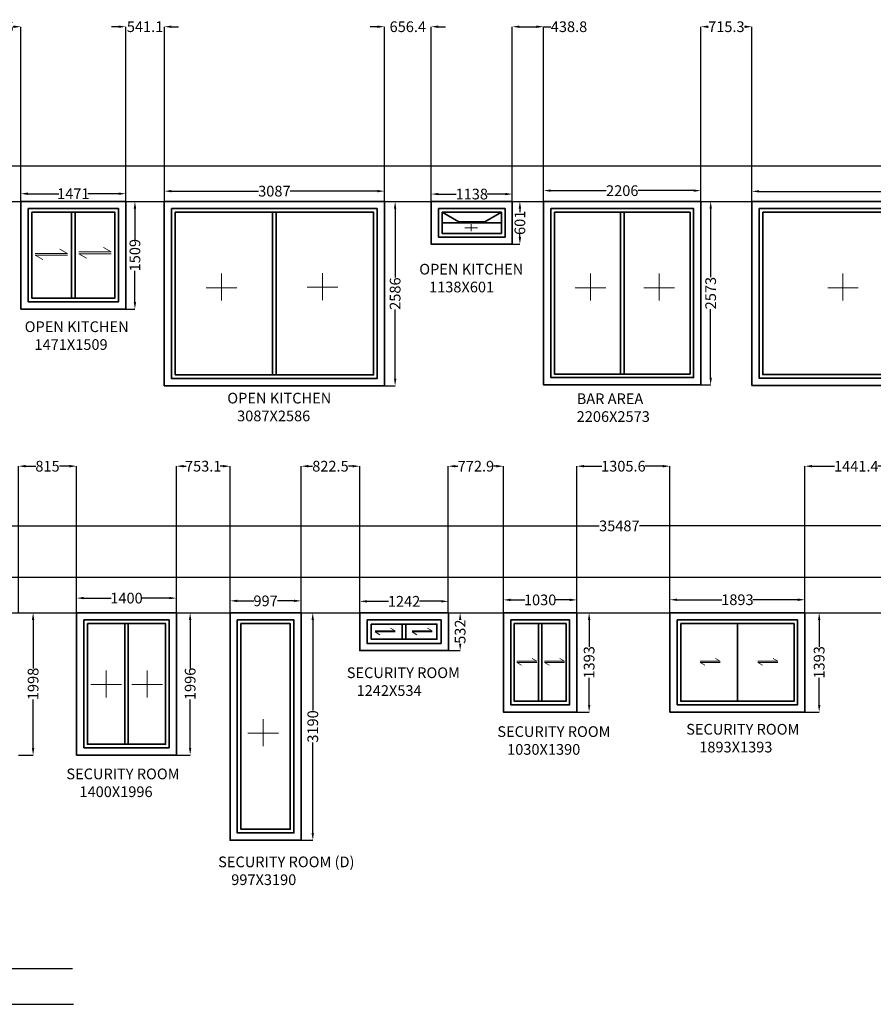
# Model space of a CAD drawing. Units: millimetres. Extents: x 16338 to 57165, y -4429 to 26237.
# Tile 5 of 6: x 28512 to 40486, y 12430 to 26237. Entities that reach past the tile are written whole.
import ezdxf

# ---------------------------------------------------------------- set-up
doc = ezdxf.new("R2010")
doc.units = ezdxf.units.MM
doc.header["$MEASUREMENT"] = 0
for name, color, linetype, lineweight in [('A-ANNO-DIMS', 5, 'Continuous', 18), ('A-ANNO-SYMB', 4, 'Continuous', 18), ('A-ANNO-TEXT', 3, 'Continuous', 18), ('A-ELEV', 8, 'Continuous', 25), ('A-GLAZ', 7, 'Continuous', 35)]:
    doc.layers.add(name, color=color, linetype=linetype, lineweight=lineweight)
doc.styles.get("Standard").update_dxf_attribs({"font": 'arial.ttf'})
doc.dimstyles.get("Standard").update_dxf_attribs({"dimtxt": 150, "dimasz": 100, "dimexe": 0.18, "dimexo": 0.0625, "dimgap": 0.09, "dimtad": 0, "dimdec": 0, "dimzin": 0, "dimdsep": 46, "dimtxsty": 'Standard', "dimcen": 0.09, "dimadec": 0, "dimazin": 0, "dimtfac": 1, "dimtdec": 0, "dimtofl": 0, "dimtmove": 0, "dimatfit": 3, "dimfxl": 1, "dimtolj": 1, "dimtzin": 0, "dimarcsym": 0})

# ---------------------------------------------------------------- blocks, each defined once
blk = doc.blocks.new('*D6')
at = {"layer": 'A-ANNO-DIMS', "color": 0, "lineweight": -2, "transparency": 16777216}
for p, q in [((28528, 23689), (28528, 23797)), ((28628, 23797), (29061, 23797)), ((29899, 23797), (29466, 23797)), ((29999, 23689), (29999, 23797))]:
    blk.add_line(p, q, dxfattribs=at)
at = {"layer": 'A-ANNO-DIMS', "color": 0, "transparency": 16777216}
for points in [[(28628, 23814), (28628, 23780), (28528, 23797)], [(29899, 23814), (29899, 23780), (29999, 23797)]]:
    blk.add_solid(points, dxfattribs=at)
at = {"layer": 'Defpoints', "color": 0, "transparency": 16777216}
for p in [(29999, 23797), (28528, 23689), (29999, 23689)]:
    blk.add_point(p, dxfattribs=at)
at = {"layer": 'A-ANNO-DIMS', "color": 0, "transparency": 16777216, "insert": (29264, 23797), "char_height": 150, "attachment_point": 5}
blk.add_mtext('\\A1;1471', dxfattribs=at)
blk = doc.blocks.new('*D7')
at = {"layer": 'A-ANNO-DIMS', "color": 0, "lineweight": -2, "transparency": 16777216}
for p, q in [((29999, 23689), (30128, 23689)), ((30128, 23589), (30128, 23152)), ((30128, 22280), (30128, 22717)), ((29999, 22180), (30128, 22180))]:
    blk.add_line(p, q, dxfattribs=at)
at = {"layer": 'A-ANNO-DIMS', "color": 0, "transparency": 16777216}
for points in [[(30111, 23589), (30145, 23589), (30128, 23689)], [(30111, 22280), (30145, 22280), (30128, 22180)]]:
    blk.add_solid(points, dxfattribs=at)
at = {"layer": 'Defpoints', "color": 0, "transparency": 16777216}
for p in [(29999, 23689), (29999, 22180), (30128, 22180)]:
    blk.add_point(p, dxfattribs=at)
at = {"layer": 'A-ANNO-DIMS', "color": 0, "transparency": 16777216, "insert": (30128, 22935), "char_height": 150, "attachment_point": 5, "rotation": 90}
blk.add_mtext('\\A1;1509', dxfattribs=at)
blk = doc.blocks.new('*D8')
at = {"layer": 'A-ANNO-DIMS', "color": 0, "lineweight": -2, "transparency": 16777216}
for p, q in [((30541, 23689), (30541, 23833)), ((30641, 23833), (31860, 23833)), ((33528, 23833), (32308, 23833)), ((33628, 23689), (33628, 23833))]:
    blk.add_line(p, q, dxfattribs=at)
at = {"layer": 'A-ANNO-DIMS', "color": 0, "transparency": 16777216}
for points in [[(30641, 23850), (30641, 23816), (30541, 23833)], [(33528, 23850), (33528, 23816), (33628, 23833)]]:
    blk.add_solid(points, dxfattribs=at)
at = {"layer": 'Defpoints', "color": 0, "transparency": 16777216}
for p in [(33628, 23833), (30541, 23689), (33628, 23689)]:
    blk.add_point(p, dxfattribs=at)
at = {"layer": 'A-ANNO-DIMS', "color": 0, "transparency": 16777216, "insert": (32084, 23833), "char_height": 150, "attachment_point": 5}
blk.add_mtext('\\A1;3087', dxfattribs=at)
blk = doc.blocks.new('*D9')
at = {"layer": 'A-ANNO-DIMS', "color": 0, "lineweight": -2, "transparency": 16777216}
for p, q in [((33628, 23689), (33779, 23689)), ((33778, 23589), (33778, 22621)), ((33778, 21203), (33778, 22171)), ((33628, 21103), (33779, 21103))]:
    blk.add_line(p, q, dxfattribs=at)
at = {"layer": 'A-ANNO-DIMS', "color": 0, "transparency": 16777216}
for points in [[(33762, 23589), (33795, 23589), (33778, 23689)], [(33762, 21203), (33795, 21203), (33778, 21103)]]:
    blk.add_solid(points, dxfattribs=at)
at = {"layer": 'Defpoints', "color": 0, "transparency": 16777216}
for p in [(33628, 23689), (33628, 21103), (33778, 21103)]:
    blk.add_point(p, dxfattribs=at)
at = {"layer": 'A-ANNO-DIMS', "color": 0, "transparency": 16777216, "insert": (33778, 22396), "char_height": 150, "attachment_point": 5, "rotation": 90}
blk.add_mtext('\\A1;2586', dxfattribs=at)
blk = doc.blocks.new('*D10')
at = {"layer": 'A-ANNO-DIMS', "color": 0, "lineweight": -2, "transparency": 16777216}
for p, q in [((34284, 23689), (34284, 23792)), ((34384, 23792), (34636, 23792)), ((35322, 23792), (35070, 23792)), ((35422, 23689), (35422, 23792))]:
    blk.add_line(p, q, dxfattribs=at)
at = {"layer": 'A-ANNO-DIMS', "color": 0, "transparency": 16777216}
for points in [[(34384, 23809), (34384, 23775), (34284, 23792)], [(35322, 23809), (35322, 23775), (35422, 23792)]]:
    blk.add_solid(points, dxfattribs=at)
at = {"layer": 'Defpoints', "color": 0, "transparency": 16777216}
for p in [(35422, 23792), (34284, 23689), (35422, 23689)]:
    blk.add_point(p, dxfattribs=at)
at = {"layer": 'A-ANNO-DIMS', "color": 0, "transparency": 16777216, "insert": (34853, 23792), "char_height": 150, "attachment_point": 5}
blk.add_mtext('\\A1;1138', dxfattribs=at)
blk = doc.blocks.new('*D11')
at = {"layer": 'A-ANNO-DIMS', "color": 0, "lineweight": -2, "transparency": 16777216}
for p, q in [((35422, 23689), (35528, 23689)), ((35528, 23589), (35528, 23540)), ((35528, 23188), (35528, 23237)), ((35422, 23088), (35528, 23088))]:
    blk.add_line(p, q, dxfattribs=at)
at = {"layer": 'A-ANNO-DIMS', "color": 0, "transparency": 16777216}
for points in [[(35511, 23589), (35545, 23589), (35528, 23689)], [(35511, 23188), (35545, 23188), (35528, 23088)]]:
    blk.add_solid(points, dxfattribs=at)
at = {"layer": 'Defpoints', "color": 0, "transparency": 16777216}
for p in [(35422, 23689), (35422, 23088), (35528, 23088)]:
    blk.add_point(p, dxfattribs=at)
at = {"layer": 'A-ANNO-DIMS', "color": 0, "transparency": 16777216, "insert": (35528, 23389), "char_height": 150, "attachment_point": 5, "rotation": 90}
blk.add_mtext('\\A1;601', dxfattribs=at)
blk = doc.blocks.new('*D12')
at = {"layer": 'A-ANNO-DIMS', "color": 0, "lineweight": -2, "transparency": 16777216}
for p, q in [((35861, 23689), (35861, 23840)), ((35961, 23840), (36738, 23840)), ((37967, 23840), (37189, 23840)), ((38067, 23689), (38067, 23840))]:
    blk.add_line(p, q, dxfattribs=at)
at = {"layer": 'A-ANNO-DIMS', "color": 0, "transparency": 16777216}
for points in [[(35961, 23857), (35961, 23824), (35861, 23840)], [(37967, 23857), (37967, 23824), (38067, 23840)]]:
    blk.add_solid(points, dxfattribs=at)
at = {"layer": 'Defpoints', "color": 0, "transparency": 16777216}
for p in [(38067, 23840), (35861, 23689), (38067, 23689)]:
    blk.add_point(p, dxfattribs=at)
at = {"layer": 'A-ANNO-DIMS', "color": 0, "transparency": 16777216, "insert": (36964, 23840), "char_height": 150, "attachment_point": 5}
blk.add_mtext('\\A1;2206', dxfattribs=at)
blk = doc.blocks.new('*D13')
at = {"layer": 'A-ANNO-DIMS', "color": 0, "lineweight": -2, "transparency": 16777216}
for p, q in [((38067, 23689), (38205, 23689)), ((38204, 23589), (38204, 22628)), ((38204, 21216), (38204, 22177)), ((38067, 21116), (38205, 21116))]:
    blk.add_line(p, q, dxfattribs=at)
at = {"layer": 'A-ANNO-DIMS', "color": 0, "transparency": 16777216}
for points in [[(38188, 23589), (38221, 23589), (38204, 23689)], [(38188, 21216), (38221, 21216), (38204, 21116)]]:
    blk.add_solid(points, dxfattribs=at)
at = {"layer": 'Defpoints', "color": 0, "transparency": 16777216}
for p in [(38067, 23689), (38067, 21116), (38204, 21116)]:
    blk.add_point(p, dxfattribs=at)
at = {"layer": 'A-ANNO-DIMS', "color": 0, "transparency": 16777216, "insert": (38204, 22403), "char_height": 150, "attachment_point": 5, "rotation": 90}
blk.add_mtext('\\A1;2573', dxfattribs=at)
blk = doc.blocks.new('*D14')
at = {"layer": 'A-ANNO-DIMS', "color": 0, "lineweight": -2, "transparency": 16777216}
for p, q in [((38782, 23689), (38782, 23831)), ((38882, 23830), (41002, 23830)), ((43575, 23830), (41456, 23830)), ((43675, 23689), (43675, 23831))]:
    blk.add_line(p, q, dxfattribs=at)
at = {"layer": 'A-ANNO-DIMS', "color": 0, "transparency": 16777216}
for points in [[(38882, 23847), (38882, 23814), (38782, 23830)], [(43575, 23847), (43575, 23814), (43675, 23830)]]:
    blk.add_solid(points, dxfattribs=at)
at = {"layer": 'Defpoints', "color": 0, "transparency": 16777216}
for p in [(43675, 23830), (38782, 23689), (43675, 23689)]:
    blk.add_point(p, dxfattribs=at)
at = {"layer": 'A-ANNO-DIMS', "color": 0, "transparency": 16777216, "insert": (41229, 23830), "char_height": 150, "attachment_point": 5}
blk.add_mtext('\\A1;4893', dxfattribs=at)
blk = doc.blocks.new('*D25')
at = {"layer": 'A-ANNO-DIMS', "color": 0, "lineweight": -2, "transparency": 16777216}
for p, q in [((28495, 17921), (28700, 17921)), ((28700, 17821), (28700, 17139)), ((28700, 16023), (28700, 16705)), ((28495, 15923), (28700, 15923))]:
    blk.add_line(p, q, dxfattribs=at)
at = {"layer": 'A-ANNO-DIMS', "color": 0, "transparency": 16777216}
for points in [[(28683, 17821), (28717, 17821), (28700, 17921)], [(28683, 16023), (28717, 16023), (28700, 15923)]]:
    blk.add_solid(points, dxfattribs=at)
at = {"layer": 'Defpoints', "color": 0, "transparency": 16777216}
for p in [(28495, 17921), (28495, 15923), (28700, 15923)]:
    blk.add_point(p, dxfattribs=at)
at = {"layer": 'A-ANNO-DIMS', "color": 0, "transparency": 16777216, "insert": (28700, 16922), "char_height": 150, "attachment_point": 5, "rotation": 90}
blk.add_mtext('\\A1;1998', dxfattribs=at)
blk = doc.blocks.new('*D26')
at = {"layer": 'A-ANNO-DIMS', "color": 0, "lineweight": -2, "transparency": 16777216}
for p, q in [((29310, 17921), (29310, 18127)), ((29410, 18126), (29793, 18126)), ((30610, 18126), (30227, 18126)), ((30710, 17921), (30710, 18127))]:
    blk.add_line(p, q, dxfattribs=at)
at = {"layer": 'A-ANNO-DIMS', "color": 0, "transparency": 16777216}
for points in [[(29410, 18143), (29410, 18110), (29310, 18126)], [(30610, 18143), (30610, 18110), (30710, 18126)]]:
    blk.add_solid(points, dxfattribs=at)
at = {"layer": 'Defpoints', "color": 0, "transparency": 16777216}
for p in [(30710, 18126), (29310, 17921), (30710, 17921)]:
    blk.add_point(p, dxfattribs=at)
at = {"layer": 'A-ANNO-DIMS', "color": 0, "transparency": 16777216, "insert": (30010, 18126), "char_height": 150, "attachment_point": 5}
blk.add_mtext('\\A1;1400', dxfattribs=at)
blk = doc.blocks.new('*D27')
at = {"layer": 'A-ANNO-DIMS', "color": 0, "lineweight": -2, "transparency": 16777216}
for p, q in [((30710, 17921), (30903, 17921)), ((30903, 17821), (30903, 17140)), ((30903, 16025), (30903, 16706)), ((30710, 15925), (30903, 15925))]:
    blk.add_line(p, q, dxfattribs=at)
at = {"layer": 'A-ANNO-DIMS', "color": 0, "transparency": 16777216}
for points in [[(30886, 17821), (30919, 17821), (30903, 17921)], [(30886, 16025), (30919, 16025), (30903, 15925)]]:
    blk.add_solid(points, dxfattribs=at)
at = {"layer": 'Defpoints', "color": 0, "transparency": 16777216}
for p in [(30710, 17921), (30710, 15925), (30903, 15925)]:
    blk.add_point(p, dxfattribs=at)
at = {"layer": 'A-ANNO-DIMS', "color": 0, "transparency": 16777216, "insert": (30903, 16923), "char_height": 150, "attachment_point": 5, "rotation": 90}
blk.add_mtext('\\A1;1996', dxfattribs=at)
blk = doc.blocks.new('*D28')
at = {"layer": 'A-ANNO-DIMS', "color": 0, "lineweight": -2, "transparency": 16777216}
for p, q in [((31463, 17921), (31463, 18087)), ((31563, 18087), (31796, 18087)), ((32360, 18087), (32127, 18087)), ((32460, 17921), (32460, 18087))]:
    blk.add_line(p, q, dxfattribs=at)
at = {"layer": 'A-ANNO-DIMS', "color": 0, "transparency": 16777216}
for points in [[(31563, 18104), (31563, 18071), (31463, 18087)], [(32360, 18104), (32360, 18071), (32460, 18087)]]:
    blk.add_solid(points, dxfattribs=at)
at = {"layer": 'Defpoints', "color": 0, "transparency": 16777216}
for p in [(32460, 18087), (31463, 17921), (32460, 17921)]:
    blk.add_point(p, dxfattribs=at)
at = {"layer": 'A-ANNO-DIMS', "color": 0, "transparency": 16777216, "insert": (31961, 18087), "char_height": 150, "attachment_point": 5}
blk.add_mtext('\\A1;997', dxfattribs=at)
blk = doc.blocks.new('*D29')
at = {"layer": 'A-ANNO-DIMS', "color": 0, "lineweight": -2, "transparency": 16777216}
for p, q in [((32460, 17921), (32623, 17921)), ((32623, 17821), (32623, 16550)), ((32623, 14831), (32623, 16102)), ((32460, 14731), (32623, 14731))]:
    blk.add_line(p, q, dxfattribs=at)
at = {"layer": 'A-ANNO-DIMS', "color": 0, "transparency": 16777216}
for points in [[(32606, 17821), (32639, 17821), (32623, 17921)], [(32606, 14831), (32639, 14831), (32623, 14731)]]:
    blk.add_solid(points, dxfattribs=at)
at = {"layer": 'Defpoints', "color": 0, "transparency": 16777216}
for p in [(32460, 17921), (32460, 14731), (32623, 14731)]:
    blk.add_point(p, dxfattribs=at)
at = {"layer": 'A-ANNO-DIMS', "color": 0, "transparency": 16777216, "insert": (32623, 16326), "char_height": 150, "attachment_point": 5, "rotation": 90}
blk.add_mtext('\\A1;3190', dxfattribs=at)
blk = doc.blocks.new('*D30')
at = {"layer": 'A-ANNO-DIMS', "color": 0, "lineweight": -2, "transparency": 16777216}
for p, q in [((33282, 17921), (33282, 18081)), ((33382, 18081), (33687, 18081)), ((34424, 18081), (34120, 18081)), ((34524, 17921), (34524, 18081))]:
    blk.add_line(p, q, dxfattribs=at)
at = {"layer": 'A-ANNO-DIMS', "color": 0, "transparency": 16777216}
for points in [[(33382, 18097), (33382, 18064), (33282, 18081)], [(34424, 18097), (34424, 18064), (34524, 18081)]]:
    blk.add_solid(points, dxfattribs=at)
at = {"layer": 'Defpoints', "color": 0, "transparency": 16777216}
for p in [(34524, 18081), (33282, 17921), (34524, 17921)]:
    blk.add_point(p, dxfattribs=at)
at = {"layer": 'A-ANNO-DIMS', "color": 0, "transparency": 16777216, "insert": (33903, 18081), "char_height": 150, "attachment_point": 5}
blk.add_mtext('\\A1;1242', dxfattribs=at)
blk = doc.blocks.new('*D31')
at = {"layer": 'A-ANNO-DIMS', "color": 0, "lineweight": -2, "transparency": 16777216}
for p, q in [((34525, 17921), (34690, 17921)), ((34690, 17821), (34690, 17820)), ((34690, 17489), (34690, 17490)), ((34525, 17389), (34690, 17389))]:
    blk.add_line(p, q, dxfattribs=at)
at = {"layer": 'A-ANNO-DIMS', "color": 0, "transparency": 16777216}
for points in [[(34674, 17821), (34707, 17821), (34690, 17921)], [(34674, 17489), (34707, 17489), (34690, 17389)]]:
    blk.add_solid(points, dxfattribs=at)
at = {"layer": 'Defpoints', "color": 0, "transparency": 16777216}
for p in [(34524, 17921), (34524, 17389), (34690, 17389)]:
    blk.add_point(p, dxfattribs=at)
at = {"layer": 'A-ANNO-DIMS', "color": 0, "transparency": 16777216, "insert": (34690, 17655), "char_height": 150, "attachment_point": 5, "rotation": 90}
blk.add_mtext('\\A1;532', dxfattribs=at)
blk = doc.blocks.new('*D32')
at = {"layer": 'A-ANNO-DIMS', "color": 0, "lineweight": -2, "transparency": 16777216}
for p, q in [((35297, 17921), (35297, 18101)), ((35397, 18101), (35596, 18101)), ((36227, 18101), (36029, 18101)), ((36327, 17921), (36327, 18101))]:
    blk.add_line(p, q, dxfattribs=at)
at = {"layer": 'A-ANNO-DIMS', "color": 0, "transparency": 16777216}
for points in [[(35397, 18118), (35397, 18084), (35297, 18101)], [(36227, 18118), (36227, 18084), (36327, 18101)]]:
    blk.add_solid(points, dxfattribs=at)
at = {"layer": 'Defpoints', "color": 0, "transparency": 16777216}
for p in [(36327, 18101), (35297, 17921), (36327, 17921)]:
    blk.add_point(p, dxfattribs=at)
at = {"layer": 'A-ANNO-DIMS', "color": 0, "transparency": 16777216, "insert": (35812, 18101), "char_height": 150, "attachment_point": 5}
blk.add_mtext('\\A1;1030', dxfattribs=at)
blk = doc.blocks.new('*D33')
at = {"layer": 'A-ANNO-DIMS', "color": 0, "lineweight": -2, "transparency": 16777216}
for p, q in [((36327, 17921), (36500, 17921)), ((36499, 17821), (36499, 17442)), ((36499, 16628), (36499, 17008)), ((36327, 16528), (36500, 16528))]:
    blk.add_line(p, q, dxfattribs=at)
at = {"layer": 'A-ANNO-DIMS', "color": 0, "transparency": 16777216}
for points in [[(36483, 17821), (36516, 17821), (36499, 17921)], [(36483, 16628), (36516, 16628), (36499, 16528)]]:
    blk.add_solid(points, dxfattribs=at)
at = {"layer": 'Defpoints', "color": 0, "transparency": 16777216}
for p in [(36327, 17921), (36327, 16528), (36499, 16528)]:
    blk.add_point(p, dxfattribs=at)
at = {"layer": 'A-ANNO-DIMS', "color": 0, "transparency": 16777216, "insert": (36499, 17225), "char_height": 150, "attachment_point": 5, "rotation": 90}
blk.add_mtext('\\A1;1393', dxfattribs=at)
blk = doc.blocks.new('*D34')
at = {"layer": 'A-ANNO-DIMS', "color": 0, "lineweight": -2, "transparency": 16777216}
for p, q in [((37633, 17921), (37633, 18103)), ((37733, 18103), (38362, 18103)), ((39426, 18103), (38796, 18103)), ((39526, 17921), (39526, 18103))]:
    blk.add_line(p, q, dxfattribs=at)
at = {"layer": 'A-ANNO-DIMS', "color": 0, "transparency": 16777216}
for points in [[(37733, 18120), (37733, 18086), (37633, 18103)], [(39426, 18120), (39426, 18086), (39526, 18103)]]:
    blk.add_solid(points, dxfattribs=at)
at = {"layer": 'Defpoints', "color": 0, "transparency": 16777216}
for p in [(39526, 18103), (37633, 17921), (39526, 17921)]:
    blk.add_point(p, dxfattribs=at)
at = {"layer": 'A-ANNO-DIMS', "color": 0, "transparency": 16777216, "insert": (38579, 18103), "char_height": 150, "attachment_point": 5}
blk.add_mtext('\\A1;1893', dxfattribs=at)
blk = doc.blocks.new('*D35')
at = {"layer": 'A-ANNO-DIMS', "color": 0, "lineweight": -2, "transparency": 16777216}
for p, q in [((39526, 17921), (39726, 17921)), ((39726, 17821), (39726, 17442)), ((39726, 16628), (39726, 17008)), ((39526, 16528), (39726, 16528))]:
    blk.add_line(p, q, dxfattribs=at)
at = {"layer": 'A-ANNO-DIMS', "color": 0, "transparency": 16777216}
for points in [[(39710, 17821), (39743, 17821), (39726, 17921)], [(39710, 16628), (39743, 16628), (39726, 16528)]]:
    blk.add_solid(points, dxfattribs=at)
at = {"layer": 'Defpoints', "color": 0, "transparency": 16777216}
for p in [(39526, 17921), (39526, 16528), (39726, 16528)]:
    blk.add_point(p, dxfattribs=at)
at = {"layer": 'A-ANNO-DIMS', "color": 0, "transparency": 16777216, "insert": (39726, 17225), "char_height": 150, "attachment_point": 5, "rotation": 90}
blk.add_mtext('\\A1;1393', dxfattribs=at)
blk = doc.blocks.new('SLIDE-ARROW-L')
for p, q in [((454, 0), (347, 62)), ((0, 0), (454, 0))]:
    blk.add_line(p, q)
blk = doc.blocks.new('SLIDE-ARROW-M')
for p, q in [((0, 0), (281, 0)), ((281, 0), (215, 38))]:
    blk.add_line(p, q)
blk = doc.blocks.new('*D84')
at = {"layer": 'A-ANNO-DIMS', "color": 0, "lineweight": -2, "transparency": 16777216}
for p, q in [((27982, 23689), (27982, 26139)), ((28082, 26139), (28090, 26139)), ((28428, 26139), (28421, 26139)), ((28528, 23689), (28528, 26139))]:
    blk.add_line(p, q, dxfattribs=at)
at = {"layer": 'A-ANNO-DIMS', "color": 0, "transparency": 16777216}
for points in [[(28082, 26156), (28082, 26122), (27982, 26139)], [(28428, 26156), (28428, 26122), (28528, 26139)]]:
    blk.add_solid(points, dxfattribs=at)
at = {"layer": 'Defpoints', "color": 0, "transparency": 16777216}
for p in [(28528, 26139), (27982, 23689), (28528, 23689)]:
    blk.add_point(p, dxfattribs=at)
at = {"layer": 'A-ANNO-DIMS', "color": 0, "transparency": 16777216, "insert": (28255, 26139), "char_height": 150, "attachment_point": 5}
blk.add_mtext('\\A1;546', dxfattribs=at)
blk = doc.blocks.new('*D85')
at = {"layer": 'A-ANNO-DIMS', "color": 0, "lineweight": -2, "transparency": 16777216}
for p, q in [((29899, 26139), (29799, 26139)), ((29999, 23689), (29999, 26139)), ((30541, 23689), (30541, 26139)), ((30641, 26139), (30741, 26139))]:
    blk.add_line(p, q, dxfattribs=at)
at = {"layer": 'A-ANNO-DIMS', "color": 0, "transparency": 16777216}
for points in [[(29899, 26156), (29899, 26122), (29999, 26139)], [(30641, 26156), (30641, 26122), (30541, 26139)]]:
    blk.add_solid(points, dxfattribs=at)
at = {"layer": 'Defpoints', "color": 0, "transparency": 16777216}
for p in [(30541, 26139), (29999, 23689), (30541, 23689)]:
    blk.add_point(p, dxfattribs=at)
at = {"layer": 'A-ANNO-DIMS', "color": 0, "transparency": 16777216, "insert": (30270, 26139), "char_height": 150, "attachment_point": 5}
blk.add_mtext('\\A1;541.1', dxfattribs=at)
blk = doc.blocks.new('*D86')
at = {"layer": 'A-ANNO-DIMS', "color": 0, "lineweight": -2, "transparency": 16777216}
for p, q in [((33528, 26139), (33428, 26139)), ((33628, 23689), (33628, 26139)), ((34284, 23689), (34284, 26139)), ((34384, 26139), (34484, 26139))]:
    blk.add_line(p, q, dxfattribs=at)
at = {"layer": 'A-ANNO-DIMS', "color": 0, "transparency": 16777216}
for points in [[(33528, 26156), (33528, 26122), (33628, 26139)], [(34384, 26156), (34384, 26122), (34284, 26139)]]:
    blk.add_solid(points, dxfattribs=at)
at = {"layer": 'Defpoints', "color": 0, "transparency": 16777216}
for p in [(34284, 26139), (33628, 23689), (34284, 23689)]:
    blk.add_point(p, dxfattribs=at)
at = {"layer": 'A-ANNO-DIMS', "color": 0, "transparency": 16777216, "insert": (33956, 26139), "char_height": 150, "attachment_point": 5}
blk.add_mtext('\\A1;656.4', dxfattribs=at)
blk = doc.blocks.new('*D87')
at = {"layer": 'A-ANNO-DIMS', "color": 0, "lineweight": -2, "transparency": 16777216}
for p, q in [((35422, 23689), (35422, 26139)), ((35522, 26139), (35761, 26139)), ((35861, 23689), (35861, 26139)), ((35861, 26139), (35961, 26139))]:
    blk.add_line(p, q, dxfattribs=at)
at = {"layer": 'A-ANNO-DIMS', "color": 0, "transparency": 16777216}
for points in [[(35522, 26156), (35522, 26122), (35422, 26139)], [(35761, 26156), (35761, 26122), (35861, 26139)]]:
    blk.add_solid(points, dxfattribs=at)
at = {"layer": 'Defpoints', "color": 0, "transparency": 16777216}
for p in [(35861, 26139), (35422, 23689), (35861, 23689)]:
    blk.add_point(p, dxfattribs=at)
at = {"layer": 'A-ANNO-DIMS', "color": 0, "transparency": 16777216, "insert": (36217, 26139), "char_height": 150, "attachment_point": 5}
blk.add_mtext('\\A1;438.8', dxfattribs=at)
blk = doc.blocks.new('*D88')
at = {"layer": 'A-ANNO-DIMS', "color": 0, "lineweight": -2, "transparency": 16777216}
for p, q in [((38067, 23689), (38067, 26139)), ((38167, 26139), (38172, 26139)), ((38682, 26139), (38677, 26139)), ((38782, 23689), (38782, 26139))]:
    blk.add_line(p, q, dxfattribs=at)
at = {"layer": 'A-ANNO-DIMS', "color": 0, "transparency": 16777216}
for points in [[(38167, 26156), (38167, 26122), (38067, 26139)], [(38682, 26156), (38682, 26122), (38782, 26139)]]:
    blk.add_solid(points, dxfattribs=at)
at = {"layer": 'Defpoints', "color": 0, "transparency": 16777216}
for p in [(38782, 26139), (38067, 23689), (38782, 23689)]:
    blk.add_point(p, dxfattribs=at)
at = {"layer": 'A-ANNO-DIMS', "color": 0, "transparency": 16777216, "insert": (38424, 26139), "char_height": 150, "attachment_point": 5}
blk.add_mtext('\\A1;715.3', dxfattribs=at)
blk = doc.blocks.new('*D91')
at = {"layer": 'A-ANNO-DIMS', "color": 0, "lineweight": -2, "transparency": 16777216}
for p, q in [((19179, 21089), (19179, 19139)), ((54667, 21100), (54667, 19139)), ((19279, 19139), (36641, 19139)), ((54567, 19139), (37205, 19139))]:
    blk.add_line(p, q, dxfattribs=at)
at = {"layer": 'A-ANNO-DIMS', "color": 0, "transparency": 16777216}
for points in [[(19279, 19156), (19279, 19122), (19179, 19139)], [(54567, 19156), (54567, 19122), (54667, 19139)]]:
    blk.add_solid(points, dxfattribs=at)
at = {"layer": 'Defpoints', "color": 0, "transparency": 16777216}
for p in [(19179, 21089), (54667, 21100), (54667, 19139)]:
    blk.add_point(p, dxfattribs=at)
at = {"layer": 'A-ANNO-DIMS', "color": 0, "transparency": 16777216, "insert": (36923, 19139), "char_height": 150, "attachment_point": 5}
blk.add_mtext('\\A1;35487', dxfattribs=at)
blk = doc.blocks.new('*D97')
at = {"layer": 'A-ANNO-DIMS', "color": 0, "lineweight": -2, "transparency": 16777216}
for p, q in [((28495, 17921), (28495, 19976)), ((28595, 19976), (28736, 19976)), ((29210, 19976), (29069, 19976)), ((29310, 17921), (29310, 19976))]:
    blk.add_line(p, q, dxfattribs=at)
at = {"layer": 'A-ANNO-DIMS', "color": 0, "transparency": 16777216}
for points in [[(28595, 19993), (28595, 19959), (28495, 19976)], [(29210, 19993), (29210, 19959), (29310, 19976)]]:
    blk.add_solid(points, dxfattribs=at)
at = {"layer": 'Defpoints', "color": 0, "transparency": 16777216}
for p in [(29310, 19976), (28495, 17921), (29310, 17921)]:
    blk.add_point(p, dxfattribs=at)
at = {"layer": 'A-ANNO-DIMS', "color": 0, "transparency": 16777216, "insert": (28902, 19976), "char_height": 150, "attachment_point": 5}
blk.add_mtext('\\A1;815', dxfattribs=at)
blk = doc.blocks.new('*D98')
at = {"layer": 'A-ANNO-DIMS', "color": 0, "lineweight": -2, "transparency": 16777216}
for p, q in [((30710, 17921), (30710, 19976)), ((30810, 19976), (30848, 19976)), ((31363, 19976), (31324, 19976)), ((31463, 17921), (31463, 19976))]:
    blk.add_line(p, q, dxfattribs=at)
at = {"layer": 'A-ANNO-DIMS', "color": 0, "transparency": 16777216}
for points in [[(30810, 19993), (30810, 19959), (30710, 19976)], [(31363, 19993), (31363, 19959), (31463, 19976)]]:
    blk.add_solid(points, dxfattribs=at)
at = {"layer": 'Defpoints', "color": 0, "transparency": 16777216}
for p in [(31463, 19976), (30710, 17921), (31463, 17921)]:
    blk.add_point(p, dxfattribs=at)
at = {"layer": 'A-ANNO-DIMS', "color": 0, "transparency": 16777216, "insert": (31086, 19976), "char_height": 150, "attachment_point": 5}
blk.add_mtext('\\A1;753.1', dxfattribs=at)
blk = doc.blocks.new('*D99')
at = {"layer": 'A-ANNO-DIMS', "color": 0, "lineweight": -2, "transparency": 16777216}
for p, q in [((32460, 17921), (32460, 19976)), ((32560, 19976), (32617, 19976)), ((33182, 19976), (33125, 19976)), ((33282, 17921), (33282, 19976))]:
    blk.add_line(p, q, dxfattribs=at)
at = {"layer": 'A-ANNO-DIMS', "color": 0, "transparency": 16777216}
for points in [[(32560, 19993), (32560, 19959), (32460, 19976)], [(33182, 19993), (33182, 19959), (33282, 19976)]]:
    blk.add_solid(points, dxfattribs=at)
at = {"layer": 'Defpoints', "color": 0, "transparency": 16777216}
for p in [(33282, 19976), (32460, 17921), (33282, 17921)]:
    blk.add_point(p, dxfattribs=at)
at = {"layer": 'A-ANNO-DIMS', "color": 0, "transparency": 16777216, "insert": (32871, 19976), "char_height": 150, "attachment_point": 5}
blk.add_mtext('\\A1;822.5', dxfattribs=at)
blk = doc.blocks.new('*D100')
at = {"layer": 'A-ANNO-DIMS', "color": 0, "lineweight": -2, "transparency": 16777216}
for p, q in [((34524, 17921), (34524, 19976)), ((34624, 19976), (34658, 19976)), ((35197, 19976), (35164, 19976)), ((35297, 17921), (35297, 19976))]:
    blk.add_line(p, q, dxfattribs=at)
at = {"layer": 'A-ANNO-DIMS', "color": 0, "transparency": 16777216}
for points in [[(34624, 19993), (34624, 19959), (34524, 19976)], [(35197, 19993), (35197, 19959), (35297, 19976)]]:
    blk.add_solid(points, dxfattribs=at)
at = {"layer": 'Defpoints', "color": 0, "transparency": 16777216}
for p in [(35297, 19976), (34524, 17921), (35297, 17921)]:
    blk.add_point(p, dxfattribs=at)
at = {"layer": 'A-ANNO-DIMS', "color": 0, "transparency": 16777216, "insert": (34911, 19976), "char_height": 150, "attachment_point": 5}
blk.add_mtext('\\A1;772.9', dxfattribs=at)
blk = doc.blocks.new('*D101')
at = {"layer": 'A-ANNO-DIMS', "color": 0, "lineweight": -2, "transparency": 16777216}
for p, q in [((36327, 17921), (36327, 19976)), ((36427, 19976), (36676, 19976)), ((37533, 19976), (37284, 19976)), ((37633, 17921), (37633, 19976))]:
    blk.add_line(p, q, dxfattribs=at)
at = {"layer": 'A-ANNO-DIMS', "color": 0, "transparency": 16777216}
for points in [[(36427, 19993), (36427, 19959), (36327, 19976)], [(37533, 19993), (37533, 19959), (37633, 19976)]]:
    blk.add_solid(points, dxfattribs=at)
at = {"layer": 'Defpoints', "color": 0, "transparency": 16777216}
for p in [(37633, 19976), (36327, 17921), (37633, 17921)]:
    blk.add_point(p, dxfattribs=at)
at = {"layer": 'A-ANNO-DIMS', "color": 0, "transparency": 16777216, "insert": (36980, 19976), "char_height": 150, "attachment_point": 5}
blk.add_mtext('\\A1;1305.6', dxfattribs=at)
blk = doc.blocks.new('*D102')
at = {"layer": 'A-ANNO-DIMS', "color": 0, "lineweight": -2, "transparency": 16777216}
for p, q in [((39526, 17921), (39526, 19976)), ((39626, 19976), (39943, 19976)), ((40867, 19976), (40551, 19976)), ((40967, 17921), (40967, 19976))]:
    blk.add_line(p, q, dxfattribs=at)
at = {"layer": 'A-ANNO-DIMS', "color": 0, "transparency": 16777216}
for points in [[(39626, 19993), (39626, 19959), (39526, 19976)], [(40867, 19993), (40867, 19959), (40967, 19976)]]:
    blk.add_solid(points, dxfattribs=at)
at = {"layer": 'Defpoints', "color": 0, "transparency": 16777216}
for p in [(40967, 19976), (39526, 17921), (40967, 17921)]:
    blk.add_point(p, dxfattribs=at)
at = {"layer": 'A-ANNO-DIMS', "color": 0, "transparency": 16777216, "insert": (40247, 19976), "char_height": 150, "attachment_point": 5}
blk.add_mtext('\\A1;1441.4', dxfattribs=at)

msp = doc.modelspace()

# ---------------------------------------------------------------- linework, layer by layer
at = {"layer": 'A-ANNO-SYMB'}
for p, q in [((34844.98, 23272.72), (34844.98, 23368.02)), ((34755.2, 23320.41), (34934.77, 23318.85)), ((31341.61, 22298.38), (31341.61, 22676.6)), ((32760.52, 22306.39), (32760.52, 22684.62)), ((36518.06, 22298.38), (36518.06, 22676.6)), ((37480.28, 22298.38), (37480.28, 22676.6)), ((40059.91, 22298.38), (40059.91, 22676.6)), ((31127.2, 22479.47), (31556.01, 22479.47)), ((32546.11, 22487.49), (32974.93, 22487.49)), ((36303.65, 22479.47), (36732.46, 22479.47)), ((37265.87, 22479.47), (37694.69, 22479.47)), ((39845.5, 22479.47), (40274.32, 22479.47)), ((29723.16, 16732.27), (29723.16, 17110.49)), ((30300.03, 16732.27), (30300.03, 17110.49)), ((29508.75, 16913.36), (29937.56, 16913.36)), ((30085.63, 16913.36), (30514.44, 16913.36)), ((31926.8, 16049.62), (31926.8, 16427.84)), ((31712.39, 16230.71), (32141.2, 16230.71))]:
    msp.add_line(p, q, dxfattribs=at)
at = {"layer": 'A-ELEV'}
for p, q in [((18334.8, 24189.02), (57164.77, 24189.02)), ((18334.8, 23689.02), (57154.46, 23689.02)), ((18334.8, 18421.15), (49111.23, 18421.15)), ((18334.8, 17921.15), (49122.07, 17921.15)), ((18334.8, 12929.59), (29250.98, 12929.59)), ((18334.8, 12429.59), (29267.6, 12429.59))]:
    msp.add_line(p, q, dxfattribs=at)
at = {"layer": 'A-GLAZ'}
for p, q in [((29238.47, 22332.42), (29238.47, 23536.62)), ((29289.27, 22332.42), (29289.27, 23536.62)), ((32058.61, 21255.42), (32058.61, 23536.62)), ((32109.41, 21255.42), (32109.41, 23536.62)), ((34436.36, 23536.62), (34670.53, 23401.42)), ((35269.56, 23536.62), (35035.39, 23401.42)), ((36938.38, 21268.42), (36938.38, 23536.62)), ((36989.18, 21268.42), (36989.18, 23536.62)), ((34436.36, 23388.52), (35269.56, 23388.52)), ((34670.53, 23401.42), (35035.39, 23401.42)), ((29984.44, 16077.55), (29984.44, 17768.75)), ((30035.24, 16077.55), (30035.24, 17768.75)), ((33878.1, 17760.75), (33878.1, 17549.55)), ((33928.9, 17760.75), (33928.9, 17549.55)), ((35786.97, 17768.75), (35786.97, 16680.55)), ((35837.77, 17768.75), (35837.77, 16680.55)), ((38579.43, 16680.55), (38579.43, 17768.75))]:
    msp.add_line(p, q, dxfattribs=at)
for points in [[(28528.37, 23689.02), (29999.37, 23689.02), (29999.37, 22180.02), (28528.37, 22180.02)], [(30540.51, 23689.02), (33627.51, 23689.02), (33627.51, 21103.02), (30540.51, 21103.02)], [(34283.96, 23689.02), (35421.96, 23689.02), (35421.96, 23088.02), (34283.96, 23088.02)], [(35860.78, 23689.02), (38066.78, 23689.02), (38066.78, 21116.02), (35860.78, 21116.02)], [(38782.09, 23689.02), (43675.09, 23689.02), (43675.09, 21109.02), (38782.09, 21109.02)], [(28629.97, 23587.42), (29897.77, 23587.42), (29897.77, 22281.62), (28629.97, 22281.62)], [(28680.77, 23536.62), (29846.97, 23536.62), (29846.97, 22332.42), (28680.77, 22332.42)], [(30642.11, 23587.42), (33525.91, 23587.42), (33525.91, 21204.62), (30642.11, 21204.62)], [(30692.91, 23536.62), (33475.11, 23536.62), (33475.11, 21255.42), (30692.91, 21255.42)], [(34385.56, 23587.42), (35320.36, 23587.42), (35320.36, 23189.62), (34385.56, 23189.62)], [(34436.36, 23536.62), (35269.56, 23536.62), (35269.56, 23240.42), (34436.36, 23240.42)], [(35962.38, 23587.42), (37965.18, 23587.42), (37965.18, 21217.62), (35962.38, 21217.62)], [(36013.18, 23536.62), (37914.38, 23536.62), (37914.38, 21268.42), (36013.18, 21268.42)], [(38883.69, 23587.42), (43573.49, 23587.42), (43573.49, 21210.62), (38883.69, 21210.62)], [(38934.49, 23536.62), (43522.69, 23536.62), (43522.69, 21261.42), (38934.49, 21261.42)], [(29309.84, 17921.15), (30709.84, 17921.15), (30709.84, 15925.15), (29309.84, 15925.15)], [(29411.44, 17819.55), (30608.24, 17819.55), (30608.24, 16026.75), (29411.44, 16026.75)], [(31462.97, 17921.15), (32459.97, 17921.15), (32459.97, 14731.15), (31462.97, 14731.15)], [(31564.57, 17819.55), (32358.37, 17819.55), (32358.37, 14832.75), (31564.57, 14832.75)], [(33282.5, 17921.15), (34524.5, 17921.15), (34524.5, 17389.15), (33282.5, 17389.15)], [(33384.1, 17819.55), (34422.9, 17819.55), (34422.9, 17490.75), (33384.1, 17490.75)], [(35297.37, 17921.15), (36327.37, 17921.15), (36327.37, 16528.15), (35297.37, 16528.15)], [(35398.97, 17819.55), (36225.77, 17819.55), (36225.77, 16629.75), (35398.97, 16629.75)], [(37632.93, 17921.15), (39525.93, 17921.15), (39525.93, 16528.15), (37632.93, 16528.15)], [(37734.53, 17819.55), (39424.33, 17819.55), (39424.33, 16629.75), (37734.53, 16629.75)], [(29462.24, 17768.75), (30557.44, 17768.75), (30557.44, 16077.55), (29462.24, 16077.55)], [(31615.37, 17768.75), (32307.57, 17768.75), (32307.57, 14883.55), (31615.37, 14883.55)], [(33442.9, 17760.75), (34364.1, 17760.75), (34364.1, 17549.55), (33442.9, 17549.55)], [(35449.77, 17768.75), (36174.97, 17768.75), (36174.97, 16680.55), (35449.77, 16680.55)], [(37785.33, 17768.75), (39373.53, 17768.75), (39373.53, 16680.55), (37785.33, 16680.55)]]:
    msp.add_lwpolyline(points, close=True, dxfattribs=at)

# ---------------------------------------------------------------- block references
at = {"layer": 'A-ANNO-SYMB'}
for name, p in [('SLIDE-ARROW-L', (28728.85, 22959.17)), ('SLIDE-ARROW-L', (29340.49, 22980.05)), ('SLIDE-ARROW-M', (33499.71, 17666.04)), ('SLIDE-ARROW-M', (34017.17, 17666.04)), ('SLIDE-ARROW-M', (35483.01, 17239.9)), ('SLIDE-ARROW-M', (35871.53, 17239.9)), ('SLIDE-ARROW-M', (38055.3, 17239.9)), ('SLIDE-ARROW-M', (38866.59, 17239.9))]:
    msp.add_blockref(name, p, dxfattribs=at)
at = {"layer": 'A-ANNO-SYMB', "rotation": 180}
for name, p in [('SLIDE-ARROW-L', (29183.05, 22934.52)), ('SLIDE-ARROW-L', (29794.69, 22955.39)), ('SLIDE-ARROW-M', (33780.69, 17650.79)), ('SLIDE-ARROW-M', (34298.14, 17650.79)), ('SLIDE-ARROW-M', (35763.99, 17224.65)), ('SLIDE-ARROW-M', (36152.5, 17224.65)), ('SLIDE-ARROW-M', (38336.27, 17224.65)), ('SLIDE-ARROW-M', (39147.56, 17224.65))]:
    msp.add_blockref(name, p, dxfattribs=at)

# ---------------------------------------------------------------- texts
at = {"layer": 'A-ANNO-TEXT', "char_height": 150, "attachment_point": 1}
for s, insert in [('OPEN KITCHEN\\P   1138X601', (34116.71, 22813.71)), ('OPEN KITCHEN\\P   1471X1509', (28581.63, 22007.03)), ('OPEN KITCHEN\\P   3087X2586', (31423.97, 21005.5)), ('BAR AREA\\P2206X2573', (36324.82, 20996.94)), ('SECURITY ROOM \\P   1242X534', (33099.84, 17154.4)), ('SECURITY ROOM \\P   1030X1390', (35211.66, 16329.03)), ('SECURITY ROOM \\P    1893X1393', (37860.97, 16361.82)), ('SECURITY ROOM \\P    1400X1996', (29166.61, 15735.48)), ('SECURITY ROOM (D)\\P    997X3190', (31295.73, 14501.93))]:
    msp.add_mtext_dynamic_manual_height_columns(s, width=7094.9176, gutter_width=1, heights=[0], dxfattribs=dict(at, insert=insert))

# ---------------------------------------------------------------- dimensions: what is measured, and where the dimension line sits
at = {"layer": 'A-ANNO-DIMS'}
for base, p1, p2, override, picture, middle in [((28528.37, 26139.02), (27982.39, 23689.02), (28528.37, 23689.02), {"dimdec": 0, "dimlfac": 1, "dimrnd": 0, "dimzin": 0, "dimdsep": 46, "dimlunit": 2}, '*D84', (28255.38, 26139.02)), ((30540.51, 26139.02), (29999.37, 23689.02), (30540.51, 23689.02), {"dimdec": 1, "dimlfac": 1, "dimrnd": 0, "dimzin": 0, "dimdsep": 46, "dimlunit": 2}, '*D85', (30269.94, 26139.02)), ((34283.9587, 26139.016), (33627.51, 23689.016), (34283.9587, 23689.016), {"dimdec": 1, "dimlfac": 1, "dimrnd": 0, "dimzin": 0, "dimdsep": 46, "dimlunit": 2}, '*D86', (33955.7344, 26139.016)), ((35860.78, 26139.02), (35421.96, 23689.02), (35860.78, 23689.02), {"dimdec": 1, "dimlfac": 1, "dimrnd": 0, "dimzin": 0, "dimdsep": 46, "dimlunit": 2}, '*D87', (36217.13, 26139.02)), ((38782.09, 26139.02), (38066.78, 23689.02), (38782.09, 23689.02), {"dimdec": 1, "dimlfac": 1, "dimrnd": 0, "dimzin": 0, "dimdsep": 46, "dimlunit": 2}, '*D88', (38424.43, 26139.02)), ((29999.37, 23797.12), (28528.37, 23689.02), (29999.37, 23689.02), {"dimclrd": 0, "dimclre": 0, "dimclrt": 0}, '*D6', (29263.87, 23797.12)), ((33627.51, 23833), (30540.51, 23689.02), (33627.51, 23689.02), {"dimclrd": 0, "dimclre": 0, "dimclrt": 0}, '*D8', (32084.01, 23833)), ((35421.96, 23791.93), (34283.96, 23689.02), (35421.96, 23689.02), {"dimclrd": 0, "dimclre": 0, "dimclrt": 0}, '*D10', (34852.96, 23791.93)), ((38066.78, 23840.28), (35860.78, 23689.02), (38066.78, 23689.02), {"dimclrd": 0, "dimclre": 0, "dimclrt": 0}, '*D12', (36963.78, 23840.28)), ((43675.09, 23830.45), (38782.09, 23689.02), (43675.09, 23689.02), {"dimclrd": 0, "dimclre": 0, "dimclrt": 0}, '*D14', (41228.59, 23830.45)), ((54666.53, 19139.02), (19179.17, 21089.02), (54666.53, 21100.02), {"dimdec": 0, "dimlfac": 1, "dimrnd": 0, "dimzin": 0, "dimdsep": 46, "dimlunit": 2}, '*D91', (36922.85, 19139.02)), ((29309.84, 19976.15), (28494.92, 17921.15), (29309.84, 17921.15), {"dimdec": 0, "dimlfac": 1, "dimrnd": 0, "dimzin": 0, "dimdsep": 46, "dimlunit": 2}, '*D97', (28902.38, 19976.15)), ((31462.97, 19976.15), (30709.84, 17921.15), (31462.97, 17921.15), {"dimdec": 1, "dimlfac": 1, "dimrnd": 0, "dimzin": 0, "dimdsep": 46, "dimlunit": 2}, '*D98', (31086.41, 19976.15)), ((33282.5, 19976.15), (32459.97, 17921.15), (33282.5, 17921.15), {"dimdec": 1, "dimlfac": 1, "dimrnd": 0, "dimzin": 0, "dimdsep": 46, "dimlunit": 2}, '*D99', (32871.23, 19976.15)), ((35297.37, 19976.15), (34524.5, 17921.15), (35297.37, 17921.15), {"dimdec": 1, "dimlfac": 1, "dimrnd": 0, "dimzin": 0, "dimdsep": 46, "dimlunit": 2}, '*D100', (34910.93, 19976.15)), ((37632.93, 19976.15), (36327.37, 17921.15), (37632.93, 17921.15), {"dimdec": 1, "dimlfac": 1, "dimrnd": 0, "dimzin": 0, "dimdsep": 46, "dimlunit": 2}, '*D101', (36980.15, 19976.15)), ((40967.34, 19976.15), (39525.93, 17921.15), (40967.34, 17921.15), {"dimdec": 1, "dimlfac": 1, "dimrnd": 0, "dimzin": 0, "dimdsep": 46, "dimlunit": 2}, '*D102', (40246.63, 19976.15)), ((30709.84, 18126.46), (29309.84, 17921.15), (30709.84, 17921.15), {"dimclrd": 0, "dimclre": 0, "dimclrt": 0}, '*D26', (30009.84, 18126.46)), ((32459.97, 18087.29), (31462.97, 17921.15), (32459.97, 17921.15), {"dimclrd": 0, "dimclre": 0, "dimclrt": 0}, '*D28', (31961.47, 18087.29)), ((34524.5, 18080.74), (33282.5, 17921.15), (34524.5, 17921.15), {"dimclrd": 0, "dimclre": 0, "dimclrt": 0}, '*D30', (33903.5, 18080.74)), ((36327.37, 18101.14), (35297.37, 17921.15), (36327.37, 17921.15), {"dimclrd": 0, "dimclre": 0, "dimclrt": 0}, '*D32', (35812.37, 18101.14)), ((39525.93, 18103.1), (37632.93, 17921.15), (39525.93, 17921.15), {"dimclrd": 0, "dimclre": 0, "dimclrt": 0}, '*D34', (38579.43, 18103.1))]:
    dim = msp.add_linear_dim(base=base, p1=p1, p2=p2, dimstyle='Standard', override=override, dxfattribs=at)
    dim.commit()
    dim.dimension.update_dxf_attribs({"geometry": picture, "text_midpoint": middle})
for base, p1, p2, picture, middle in [((30128.06, 22180.02), (29999.37, 23689.02), (29999.37, 22180.02), '*D7', (30128.06, 22934.52)), ((33778.38, 21103.02), (33627.51, 23689.02), (33627.51, 21103.02), '*D9', (33778.38, 22396.02)), ((35527.93, 23088.02), (35421.96, 23689.02), (35421.96, 23088.02), '*D11', (35527.93, 23388.52)), ((38204.43, 21116.02), (38066.78, 23689.02), (38066.78, 21116.02), '*D13', (38204.43, 22402.52)), ((28699.97, 15923.15), (28494.92, 17921.15), (28494.92, 15923.15), '*D25', (28699.97, 16922.15)), ((30902.81, 15925.15), (30709.84, 17921.15), (30709.84, 15925.15), '*D27', (30902.81, 16923.15)), ((32622.52, 14731.15), (32459.97, 17921.15), (32459.97, 14731.15), '*D29', (32622.52, 16326.15)), ((34690.22, 17389.15), (34524.5, 17921.15), (34524.5, 17389.15), '*D31', (34690.22, 17655.15)), ((36499.36, 16528.15), (36327.37, 17921.15), (36327.37, 16528.15), '*D33', (36499.36, 17224.65)), ((39726.22, 16528.15), (39525.93, 17921.15), (39525.93, 16528.15), '*D35', (39726.22, 17224.65))]:
    dim = msp.add_linear_dim(base=base, p1=p1, p2=p2, angle=90, dimstyle='Standard', override={"dimclrd": 0, "dimclre": 0, "dimclrt": 0}, dxfattribs=at)
    dim.commit()
    dim.dimension.update_dxf_attribs({"geometry": picture, "text_midpoint": middle})

doc.saveas('drawing.dxf')
